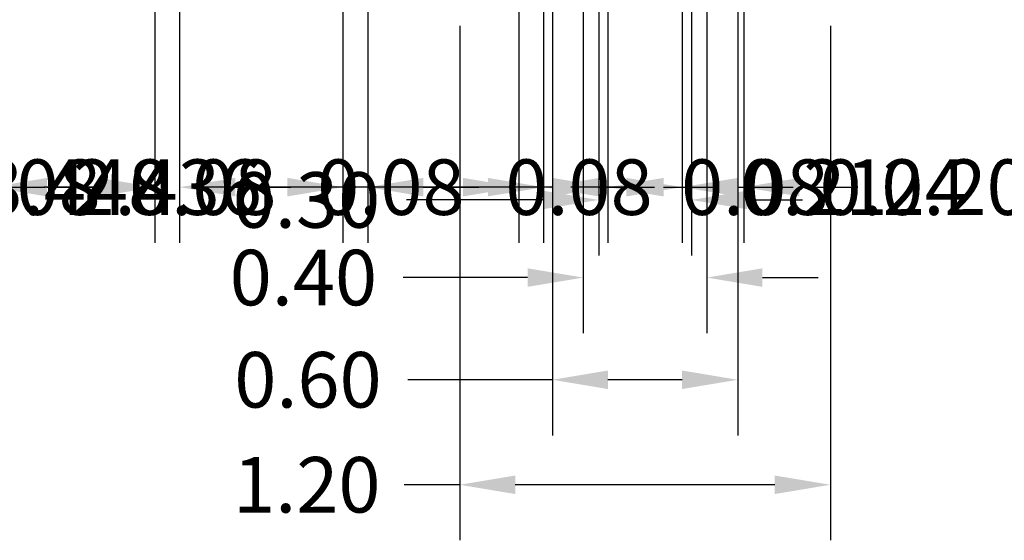
# Model space of a CAD drawing. Units: metres. Extents: x 22.1 to 34.4, y 4.4 to 12.4.
# Tile 3 of 8: x 29.6 to 32.8, y 5.3 to 7. Entities that reach past the tile are written whole.
import ezdxf

# ---------------------------------------------------------------- set-up
doc = ezdxf.new("R2010")
doc.units = ezdxf.units.M
doc.header["$MEASUREMENT"] = 0
doc.layers.add('A-ANNO-DIMS', color=2, linetype='Continuous', lineweight=18)
doc.styles.get("Standard").update_dxf_attribs({"font": 'arial.ttf'})
doc.dimstyles.get("Standard").update_dxf_attribs({"dimtxt": 0.18, "dimasz": 0.18, "dimexe": 0.18, "dimexo": 0.0625, "dimgap": 0.09, "dimtad": 0, "dimtih": 1, "dimtoh": 1, "dimzin": 0, "dimdsep": 46, "dimtxsty": 'Standard', "dimcen": 0.09, "dimadec": 0, "dimazin": 0, "dimtfac": 1, "dimtofl": 0, "dimtmove": 0, "dimatfit": 3, "dimfxl": 1, "dimtolj": 1, "dimtzin": 0, "dimarcsym": 0})

# ---------------------------------------------------------------- blocks, each defined once
blk = doc.blocks.new('*D7')
at = {"layer": 'A-ANNO-DIMS', "color": 0, "lineweight": -2, "transparency": 16777216}
for p, q in [((31.0581, 6.9474), (31.0581, 5.2806)), ((32.2581, 6.9474), (32.2581, 5.2806)), ((31.0581, 5.4606), (30.8781, 5.4606)), ((32.0781, 5.4606), (31.2381, 5.4606))]:
    blk.add_line(p, q, dxfattribs=at)
at = {"layer": 'A-ANNO-DIMS', "color": 0, "transparency": 16777216}
for points in [[(31.2381, 5.4906), (31.2381, 5.4306), (31.0581, 5.4606)], [(32.0781, 5.4906), (32.0781, 5.4306), (32.2581, 5.4606)]]:
    blk.add_solid(points, dxfattribs=at)
at = {"layer": 'Defpoints', "color": 0, "transparency": 16777216}
for p in [(31.0581, 7.0099), (32.2581, 7.0099), (32.2581, 5.4606)]:
    blk.add_point(p, dxfattribs=at)
at = {"layer": 'A-ANNO-DIMS', "color": 0, "transparency": 16777216, "insert": (30.5631, 5.4606), "char_height": 0.18, "attachment_point": 5}
blk.add_mtext('\\A1;1.20', dxfattribs=at)
blk = doc.blocks.new('*D8')
at = {"layer": 'A-ANNO-DIMS', "color": 0, "lineweight": -2, "transparency": 16777216}
for p, q in [((31.3581, 7.1474), (31.3581, 5.6208)), ((31.9581, 7.1474), (31.9581, 5.6208)), ((31.3581, 5.8008), (30.8904, 5.8008)), ((31.7781, 5.8008), (31.5381, 5.8008))]:
    blk.add_line(p, q, dxfattribs=at)
at = {"layer": 'A-ANNO-DIMS', "color": 0, "transparency": 16777216}
for points in [[(31.5381, 5.8308), (31.5381, 5.7708), (31.3581, 5.8008)], [(31.7781, 5.8308), (31.7781, 5.7708), (31.9581, 5.8008)]]:
    blk.add_solid(points, dxfattribs=at)
at = {"layer": 'Defpoints', "color": 0, "transparency": 16777216}
for p in [(31.3581, 7.2099), (31.9581, 7.2099), (31.9581, 5.8008)]:
    blk.add_point(p, dxfattribs=at)
at = {"layer": 'A-ANNO-DIMS', "color": 0, "transparency": 16777216, "insert": (30.5669, 5.8008), "char_height": 0.18, "attachment_point": 5}
blk.add_mtext('\\A1;0.60', dxfattribs=at)
blk = doc.blocks.new('*D9')
at = {"layer": 'A-ANNO-DIMS', "color": 0, "lineweight": -2, "transparency": 16777216}
for p, q in [((31.4581, 7.4974), (31.4581, 5.952)), ((31.8581, 7.4974), (31.8581, 5.952)), ((31.2781, 6.132), (30.8756, 6.132)), ((32.0381, 6.132), (32.2181, 6.132))]:
    blk.add_line(p, q, dxfattribs=at)
at = {"layer": 'A-ANNO-DIMS', "color": 0, "transparency": 16777216}
for points in [[(31.2781, 6.162), (31.2781, 6.102), (31.4581, 6.132)], [(32.0381, 6.162), (32.0381, 6.102), (31.8581, 6.132)]]:
    blk.add_solid(points, dxfattribs=at)
at = {"layer": 'Defpoints', "color": 0, "transparency": 16777216}
for p in [(31.4581, 7.5599), (31.8581, 7.5599), (31.8581, 6.132)]:
    blk.add_point(p, dxfattribs=at)
at = {"layer": 'A-ANNO-DIMS', "color": 0, "transparency": 16777216, "insert": (30.5521, 6.132), "char_height": 0.18, "attachment_point": 5}
blk.add_mtext('\\A1;0.40', dxfattribs=at)
blk = doc.blocks.new('*D10')
at = {"layer": 'A-ANNO-DIMS', "color": 0, "lineweight": -2, "transparency": 16777216}
for p, q in [((31.5081, 7.8474), (31.5081, 6.2035)), ((31.8081, 7.8474), (31.8081, 6.2035)), ((31.3281, 6.3835), (30.8854, 6.3835)), ((31.9881, 6.3835), (32.1681, 6.3835))]:
    blk.add_line(p, q, dxfattribs=at)
at = {"layer": 'A-ANNO-DIMS', "color": 0, "transparency": 16777216}
for points in [[(31.3281, 6.4135), (31.3281, 6.3535), (31.5081, 6.3835)], [(31.9881, 6.4135), (31.9881, 6.3535), (31.8081, 6.3835)]]:
    blk.add_solid(points, dxfattribs=at)
at = {"layer": 'Defpoints', "color": 0, "transparency": 16777216}
for p in [(31.5081, 7.9099), (31.8081, 7.9099), (31.8081, 6.3835)]:
    blk.add_point(p, dxfattribs=at)
at = {"layer": 'A-ANNO-DIMS', "color": 0, "transparency": 16777216, "insert": (30.562, 6.3835), "char_height": 0.18, "attachment_point": 5}
blk.add_mtext('\\A1;0.30', dxfattribs=at)
blk = doc.blocks.new('*D23')
at = {"layer": 'A-ANNO-DIMS', "color": 0, "lineweight": -2, "transparency": 16777216}
for p, q in [((28.0901, 11.4474), (28.0901, 6.2449)), ((31.5381, 11.4474), (31.5381, 6.2449)), ((28.2701, 6.4249), (29.4202, 6.4249)), ((31.3581, 6.4249), (30.2079, 6.4249))]:
    blk.add_line(p, q, dxfattribs=at)
at = {"layer": 'A-ANNO-DIMS', "color": 0, "transparency": 16777216}
for points in [[(28.2701, 6.4549), (28.2701, 6.3949), (28.0901, 6.4249)], [(31.3581, 6.4549), (31.3581, 6.3949), (31.5381, 6.4249)]]:
    blk.add_solid(points, dxfattribs=at)
at = {"layer": 'Defpoints', "color": 0, "transparency": 16777216}
for p in [(28.0901, 11.5099), (31.5381, 11.5099), (31.5381, 6.4249)]:
    blk.add_point(p, dxfattribs=at)
at = {"layer": 'A-ANNO-DIMS', "color": 0, "transparency": 16777216, "insert": (29.8141, 6.4249), "char_height": 0.18, "attachment_point": 5}
blk.add_mtext('\\A1;3.448', dxfattribs=at)
blk = doc.blocks.new('*D27')
at = {"layer": 'A-ANNO-DIMS', "color": 0, "lineweight": -2, "transparency": 16777216}
for p, q in [((31.5381, 11.4474), (31.5381, 6.2449)), ((31.7781, 11.4474), (31.7781, 6.2449)), ((31.3581, 6.4249), (31.1781, 6.4249)), ((31.9581, 6.4249), (32.1381, 6.4249))]:
    blk.add_line(p, q, dxfattribs=at)
at = {"layer": 'A-ANNO-DIMS', "color": 0, "transparency": 16777216}
for points in [[(31.3581, 6.4549), (31.3581, 6.3949), (31.5381, 6.4249)], [(31.9581, 6.4549), (31.9581, 6.3949), (31.7781, 6.4249)]]:
    blk.add_solid(points, dxfattribs=at)
at = {"layer": 'Defpoints', "color": 0, "transparency": 16777216}
for p in [(31.5381, 11.5099), (31.7781, 11.5099), (31.7781, 6.4249)]:
    blk.add_point(p, dxfattribs=at)
at = {"layer": 'A-ANNO-DIMS', "color": 0, "transparency": 16777216, "insert": (32.4615, 6.4249), "char_height": 0.18, "attachment_point": 5}
blk.add_mtext('\\A1;0.24', dxfattribs=at)
blk = doc.blocks.new('*D28')
at = {"layer": 'A-ANNO-DIMS', "color": 0, "lineweight": -2, "transparency": 16777216}
for p, q in [((31.7781, 11.4474), (31.7781, 6.2449)), ((31.9781, 11.4474), (31.9781, 6.2449)), ((31.5981, 6.4249), (31.4181, 6.4249)), ((32.1581, 6.4249), (32.3381, 6.4249))]:
    blk.add_line(p, q, dxfattribs=at)
at = {"layer": 'A-ANNO-DIMS', "color": 0, "transparency": 16777216}
for points in [[(31.5981, 6.4549), (31.5981, 6.3949), (31.7781, 6.4249)], [(32.1581, 6.4549), (32.1581, 6.3949), (31.9781, 6.4249)]]:
    blk.add_solid(points, dxfattribs=at)
at = {"layer": 'Defpoints', "color": 0, "transparency": 16777216}
for p in [(31.7781, 11.5099), (31.9781, 11.5099), (31.9781, 6.4249)]:
    blk.add_point(p, dxfattribs=at)
at = {"layer": 'A-ANNO-DIMS', "color": 0, "transparency": 16777216, "insert": (32.6615, 6.4249), "char_height": 0.18, "attachment_point": 5}
blk.add_mtext('\\A1;0.20', dxfattribs=at)
blk = doc.blocks.new('*D33')
at = {"layer": 'A-ANNO-DIMS', "color": 0, "lineweight": -2, "transparency": 16777216}
for p, q in [((31.5381, 11.4474), (31.5381, 6.2449)), ((31.3293, 10.5774), (31.3293, 6.2449)), ((31.1493, 6.4249), (30.9693, 6.4249)), ((31.7181, 6.4249), (31.8981, 6.4249))]:
    blk.add_line(p, q, dxfattribs=at)
at = {"layer": 'A-ANNO-DIMS', "color": 0, "transparency": 16777216}
for points in [[(31.1493, 6.4549), (31.1493, 6.3949), (31.3293, 6.4249)], [(31.7181, 6.4549), (31.7181, 6.3949), (31.5381, 6.4249)]]:
    blk.add_solid(points, dxfattribs=at)
at = {"layer": 'Defpoints', "color": 0, "transparency": 16777216}
for p in [(31.5381, 11.5099), (31.3293, 10.6399), (31.5381, 6.4249)]:
    blk.add_point(p, dxfattribs=at)
at = {"layer": 'A-ANNO-DIMS', "color": 0, "transparency": 16777216, "insert": (32.2045, 6.4249), "char_height": 0.18, "attachment_point": 5}
blk.add_mtext('\\A1;0.21', dxfattribs=at)
blk = doc.blocks.new('*D34')
at = {"layer": 'A-ANNO-DIMS', "color": 0, "lineweight": -2, "transparency": 16777216}
for p, q in [((28.8933, 9.3614), (28.8933, 6.2449)), ((31.3293, 9.3614), (31.3293, 6.2449)), ((29.0733, 6.4249), (29.7162, 6.4249)), ((31.1493, 6.4249), (30.5065, 6.4249))]:
    blk.add_line(p, q, dxfattribs=at)
at = {"layer": 'A-ANNO-DIMS', "color": 0, "transparency": 16777216}
for points in [[(29.0733, 6.4549), (29.0733, 6.3949), (28.8933, 6.4249)], [(31.1493, 6.4549), (31.1493, 6.3949), (31.3293, 6.4249)]]:
    blk.add_solid(points, dxfattribs=at)
at = {"layer": 'Defpoints', "color": 0, "transparency": 16777216}
for p in [(28.8933, 9.4239), (31.3293, 9.4239), (31.3293, 6.4249)]:
    blk.add_point(p, dxfattribs=at)
at = {"layer": 'A-ANNO-DIMS', "color": 0, "transparency": 16777216, "insert": (30.1113, 6.4249), "char_height": 0.18, "attachment_point": 5}
blk.add_mtext('\\A1;2.436', dxfattribs=at)
blk = doc.blocks.new('*D35')
at = {"layer": 'A-ANNO-DIMS', "color": 0, "lineweight": -2, "transparency": 16777216}
for p, q in [((28.9733, 9.4414), (28.9733, 6.2449)), ((28.8933, 9.3614), (28.8933, 6.2449)), ((28.7133, 6.4249), (28.5333, 6.4249)), ((29.1533, 6.4249), (29.3333, 6.4249))]:
    blk.add_line(p, q, dxfattribs=at)
at = {"layer": 'A-ANNO-DIMS', "color": 0, "transparency": 16777216}
for points in [[(28.7133, 6.4549), (28.7133, 6.3949), (28.8933, 6.4249)], [(29.1533, 6.4549), (29.1533, 6.3949), (28.9733, 6.4249)]]:
    blk.add_solid(points, dxfattribs=at)
at = {"layer": 'Defpoints', "color": 0, "transparency": 16777216}
for p in [(28.9733, 9.5039), (28.8933, 9.4239), (28.9733, 6.4249)]:
    blk.add_point(p, dxfattribs=at)
at = {"layer": 'A-ANNO-DIMS', "color": 0, "transparency": 16777216, "insert": (29.6573, 6.4249), "char_height": 0.18, "attachment_point": 5}
blk.add_mtext('\\A1;0.08', dxfattribs=at)
blk = doc.blocks.new('*D36')
at = {"layer": 'A-ANNO-DIMS', "color": 0, "lineweight": -2, "transparency": 16777216}
for p, q in [((29.4623, 9.4414), (29.4623, 6.2449)), ((29.5423, 9.4414), (29.5423, 6.2449)), ((29.2823, 6.4249), (29.1023, 6.4249)), ((29.7223, 6.4249), (29.9023, 6.4249))]:
    blk.add_line(p, q, dxfattribs=at)
at = {"layer": 'A-ANNO-DIMS', "color": 0, "transparency": 16777216}
for points in [[(29.2823, 6.4549), (29.2823, 6.3949), (29.4623, 6.4249)], [(29.7223, 6.4549), (29.7223, 6.3949), (29.5423, 6.4249)]]:
    blk.add_solid(points, dxfattribs=at)
at = {"layer": 'Defpoints', "color": 0, "transparency": 16777216}
for p in [(29.4623, 9.5039), (29.5423, 9.5039), (29.5423, 6.4249)]:
    blk.add_point(p, dxfattribs=at)
at = {"layer": 'A-ANNO-DIMS', "color": 0, "transparency": 16777216, "insert": (30.2263, 6.4249), "char_height": 0.18, "attachment_point": 5}
blk.add_mtext('\\A1;0.08', dxfattribs=at)
blk = doc.blocks.new('*D37')
at = {"layer": 'A-ANNO-DIMS', "color": 0, "lineweight": -2, "transparency": 16777216}
for p, q in [((30.0713, 9.4414), (30.0713, 6.2449)), ((30.1513, 9.4414), (30.1513, 6.2449)), ((29.8913, 6.4249), (29.7113, 6.4249)), ((30.3313, 6.4249), (30.5113, 6.4249))]:
    blk.add_line(p, q, dxfattribs=at)
at = {"layer": 'A-ANNO-DIMS', "color": 0, "transparency": 16777216}
for points in [[(29.8913, 6.4549), (29.8913, 6.3949), (30.0713, 6.4249)], [(30.3313, 6.4549), (30.3313, 6.3949), (30.1513, 6.4249)]]:
    blk.add_solid(points, dxfattribs=at)
at = {"layer": 'Defpoints', "color": 0, "transparency": 16777216}
for p in [(30.0713, 9.5039), (30.1513, 9.5039), (30.1513, 6.4249)]:
    blk.add_point(p, dxfattribs=at)
at = {"layer": 'A-ANNO-DIMS', "color": 0, "transparency": 16777216, "insert": (30.8353, 6.4249), "char_height": 0.18, "attachment_point": 5}
blk.add_mtext('\\A1;0.08', dxfattribs=at)
blk = doc.blocks.new('*D38')
at = {"layer": 'A-ANNO-DIMS', "color": 0, "lineweight": -2, "transparency": 16777216}
for p, q in [((30.6803, 9.4414), (30.6803, 6.2449)), ((30.7603, 9.4414), (30.7603, 6.2449)), ((30.5003, 6.4249), (30.3203, 6.4249)), ((30.9403, 6.4249), (31.1203, 6.4249))]:
    blk.add_line(p, q, dxfattribs=at)
at = {"layer": 'A-ANNO-DIMS', "color": 0, "transparency": 16777216}
for points in [[(30.5003, 6.4549), (30.5003, 6.3949), (30.6803, 6.4249)], [(30.9403, 6.4549), (30.9403, 6.3949), (30.7603, 6.4249)]]:
    blk.add_solid(points, dxfattribs=at)
at = {"layer": 'Defpoints', "color": 0, "transparency": 16777216}
for p in [(30.6803, 9.5039), (30.7603, 9.5039), (30.7603, 6.4249)]:
    blk.add_point(p, dxfattribs=at)
at = {"layer": 'A-ANNO-DIMS', "color": 0, "transparency": 16777216, "insert": (31.4443, 6.4249), "char_height": 0.18, "attachment_point": 5}
blk.add_mtext('\\A1;0.08', dxfattribs=at)
blk = doc.blocks.new('*D39')
at = {"layer": 'A-ANNO-DIMS', "color": 0, "lineweight": -2, "transparency": 16777216}
for p, q in [((31.2493, 9.4414), (31.2493, 6.2449)), ((31.3293, 9.3614), (31.3293, 6.2449)), ((31.0693, 6.4249), (30.8893, 6.4249)), ((31.5093, 6.4249), (31.6893, 6.4249))]:
    blk.add_line(p, q, dxfattribs=at)
at = {"layer": 'A-ANNO-DIMS', "color": 0, "transparency": 16777216}
for points in [[(31.0693, 6.4549), (31.0693, 6.3949), (31.2493, 6.4249)], [(31.5093, 6.4549), (31.5093, 6.3949), (31.3293, 6.4249)]]:
    blk.add_solid(points, dxfattribs=at)
at = {"layer": 'Defpoints', "color": 0, "transparency": 16777216}
for p in [(31.2493, 9.5039), (31.3293, 9.4239), (31.3293, 6.4249)]:
    blk.add_point(p, dxfattribs=at)
at = {"layer": 'A-ANNO-DIMS', "color": 0, "transparency": 16777216, "insert": (32.0133, 6.4249), "char_height": 0.18, "attachment_point": 5}
blk.add_mtext('\\A1;0.08', dxfattribs=at)

msp = doc.modelspace()

# ---------------------------------------------------------------- dimensions: what is measured, and where the dimension line sits
at = {"layer": 'A-ANNO-DIMS'}
for base, p1, p2, override, picture, middle in [((31.5381, 6.4249), (28.0901, 11.5099), (31.5381, 11.5099), {"dimdec": 3, "dimlfac": 1, "dimrnd": 0, "dimzin": 0, "dimdsep": 46, "dimlunit": 2}, '*D23', (29.8141, 6.4249)), ((31.5381, 6.4249), (31.3293, 10.6399), (31.5381, 11.5099), {"dimdec": 2, "dimlfac": 1, "dimrnd": 0, "dimzin": 0, "dimdsep": 46, "dimlunit": 2}, '*D33', (32.2045, 6.4249)), ((31.7781, 6.4249), (31.5381, 11.5099), (31.7781, 11.5099), {"dimdec": 2, "dimlfac": 1, "dimrnd": 0, "dimzin": 0, "dimdsep": 46, "dimlunit": 2}, '*D27', (32.4615, 6.4249)), ((31.9781, 6.4249), (31.7781, 11.5099), (31.9781, 11.5099), {"dimdec": 2, "dimlfac": 1, "dimrnd": 0, "dimzin": 0, "dimdsep": 46, "dimlunit": 2}, '*D28', (32.6615, 6.4249)), ((28.9733, 6.4249), (28.8933, 9.4239), (28.9733, 9.5039), {"dimdec": 2, "dimlfac": 1, "dimrnd": 0, "dimzin": 0, "dimdsep": 46, "dimlunit": 2}, '*D35', (29.6573, 6.4249)), ((29.5423, 6.4249), (29.4623, 9.5039), (29.5423, 9.5039), {"dimdec": 2, "dimlfac": 1, "dimrnd": 0, "dimzin": 0, "dimdsep": 46, "dimlunit": 2}, '*D36', (30.2263, 6.4249)), ((30.1513, 6.4249), (30.0713, 9.5039), (30.1513, 9.5039), {"dimdec": 2, "dimlfac": 1, "dimrnd": 0, "dimzin": 0, "dimdsep": 46, "dimlunit": 2}, '*D37', (30.8353, 6.4249)), ((30.7603, 6.4249), (30.6803, 9.5039), (30.7603, 9.5039), {"dimdec": 2, "dimlfac": 1, "dimrnd": 0, "dimzin": 0, "dimdsep": 46, "dimlunit": 2}, '*D38', (31.4443, 6.4249)), ((31.3293, 6.4249), (31.2493, 9.5039), (31.3293, 9.4239), {"dimdec": 2, "dimlfac": 1, "dimrnd": 0, "dimzin": 0, "dimdsep": 46, "dimlunit": 2}, '*D39', (32.0133, 6.4249)), ((31.3293, 6.4249), (28.8933, 9.4239), (31.3293, 9.4239), {"dimdec": 3, "dimlfac": 1, "dimrnd": 0, "dimzin": 0, "dimdsep": 46, "dimlunit": 2}, '*D34', (30.1113, 6.4249))]:
    dim = msp.add_linear_dim(base=base, p1=p1, p2=p2, dimstyle='Standard', override=override, dxfattribs=at)
    dim.commit()
    dim.dimension.update_dxf_attribs({"geometry": picture, "text_midpoint": middle})
for base, p1, p2, picture, middle in [((31.8081, 6.3835), (31.5081, 7.9099), (31.8081, 7.9099), '*D10', (30.562, 6.3835)), ((31.8581, 6.132), (31.4581, 7.5599), (31.8581, 7.5599), '*D9', (30.5521, 6.132)), ((31.9581, 5.8008), (31.3581, 7.2099), (31.9581, 7.2099), '*D8', (30.5669, 5.8008)), ((32.2581, 5.4606), (31.0581, 7.0099), (32.2581, 7.0099), '*D7', (30.5631, 5.4606))]:
    dim = msp.add_linear_dim(base=base, p1=p1, p2=p2, dimstyle='Standard', override={"dimclrd": 0, "dimclre": 0, "dimclrt": 0}, dxfattribs=at)
    dim.commit()
    dim.dimension.update_dxf_attribs({"geometry": picture, "text_midpoint": middle, "dimtype": 160})

doc.saveas('drawing.dxf')
